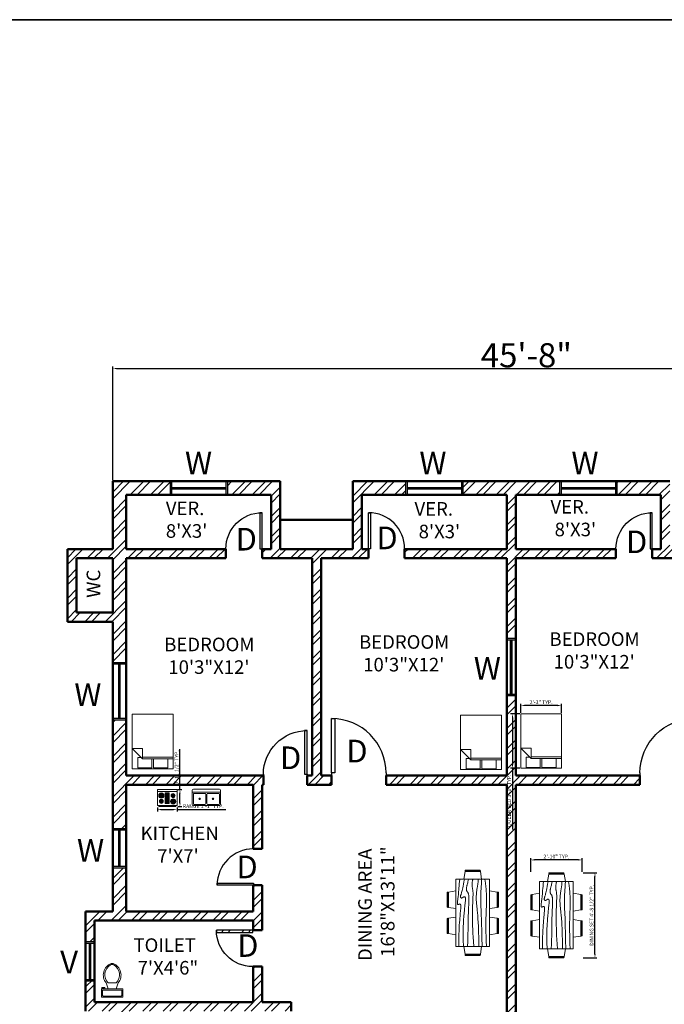
# Model space of a CAD drawing. Units: inches. Extents: x -31485 to -28799, y 18003 to 19130.
# Tile 9 of 15: x -30506 to -30079, y 18478 to 19130. Entities that reach past the tile are written whole.
import ezdxf

# ---------------------------------------------------------------- set-up
doc = ezdxf.new("R2010")
doc.units = ezdxf.units.IN
for name, color, linetype, lineweight in [('A-ANNO-DIMS', 2, 'Continuous', 18), ('A-ANNO-TEXT', 7, 'Continuous', 18), ('A-ANNO-TTLB', 7, 'Continuous', 35), ('A-AREA-IDEN', 7, 'Continuous', 18), ('A-DOOR', 3, 'Continuous', 25), ('A-FLOR-FIXT', 9, 'Continuous', 18), ('A-FURN', 8, 'Continuous', 18), ('A-GLAZ', 4, 'Continuous', 25), ('A-WALL', 7, 'Continuous', 50), ('A-WALL-PATT', 8, 'Continuous', 13)]:
    doc.layers.add(name, color=color, linetype=linetype, lineweight=lineweight)
doc.styles.get("Standard").update_dxf_attribs({"font": 'arial.ttf'})
doc.dimstyles.new('ISO-25', dxfattribs={"dimtxt": 2.5, "dimasz": 2.5, "dimexe": 1.25, "dimexo": 0.625, "dimtad": 1, "dimdec": 0, "dimlunit": 3, "dimtxsty": 'Standard', "dimcen": 2.5, "dimadec": 0, "dimazin": 0, "dimtfac": 1, "dimtdec": 0, "dimtmove": 0, "dimatfit": 3, "dimfxl": 1, "dimarcsym": 0})

# ---------------------------------------------------------------- blocks, each defined once
blk = doc.blocks.new('*U8')
for p, q in [((0, 0), (0, -100)), ((750, 0), (750, -100))]:
    blk.add_line(p, q)
blk.add_lwpolyline([(0, 0), (0, 750), (43.75, 750), (43.75, 0)], close=True)
blk.add_arc((0, 0), 750, 0, 90)
blk = doc.blocks.new('Bed - Queen')
for p, q in [((0, -80.00003), (0, 0)), ((0, 0), (59.99999, 0)), ((59.99999, 0), (59.99999, -80.00003)), ((0, -14.4), (44.8, -14.4)), ((7.99999, -1.2), (28.79998, -1.2)), ((7.99999, -14.4), (7.99999, -1.2)), ((28.79998, -1.2), (28.79998, -14.4)), ((31.19999, -1.2), (51.99999, -1.2)), ((31.19999, -14.4), (31.19999, -1.2)), ((59.99999, -29.6), (44.8, -14.4)), ((44.8, -14.4), (44.8, -29.6)), ((51.99999, -1.2), (51.99999, -16.4)), ((44.8, -16.8), (0, -16.8)), ((51.99999, -16.4), (46.79936, -16.4)), ((44.8, -29.6), (59.99999, -29.6)), ((59.99999, -80.00003), (0, -80.00003))]:
    blk.add_line(p, q)
blk = doc.blocks.new('Range-Oven - 30 in top')
for p, q in [((0, -3), (30, -3)), ((12, -6), (18, -6)), ((13, -20), (13, -6)), ((14, -6), (14, -20)), ((15, -20), (15, -6)), ((16, -6), (16, -20)), ((17, -20), (17, -6)), ((6, -24), (6, -25)), ((8, -25), (8, -24)), ((18, -20), (12, -20)), ((22, -25), (22, -24)), ((24, -24), (24, -25))]:
    blk.add_line(p, q)
for points in [[(0, -24), (0, 0), (30, 0), (30, -24)], [(12, -21), (12, -5), (18, -5), (18, -21)], [(2, -26), (2, -25), (28, -25), (28, -26)]]:
    blk.add_lwpolyline(points, close=True)
for centre, radius in [((6, -9), 4), ((6, -9), 3), ((6, -18), 3), ((6, -9), 2), ((6, -9), 1), ((24, -18), 4), ((24, -9), 3), ((24, -18), 3), ((24, -9), 2), ((24, -9), 1), ((6, -18), 2), ((6, -18), 1), ((24, -18), 2), ((24, -18), 1)]:
    blk.add_circle(centre, radius)
blk = doc.blocks.new('Sink-double - 36 in top')
for p, q in [((-18, -4), (18, -4)), ((-0.75, -18.5), (-0.75, -6.5)), ((0.75, -6.5), (0.75, -18.5))]:
    blk.add_line(p, q)
for points in [[(-16.5, 0), (16.5, 0)], [(-18, -19.5), (-18, -1.5)], [(-16.5, -18.5), (-16.5, -6.5)], [(-15.5, -5.5), (-1.75, -5.5)], [(1.75, -5.5), (15.5, -5.5)], [(16.5, -6.5), (16.5, -18.5)], [(18, -1.5), (18, -19.5)], [(16.5, -21), (-16.5, -21)], [(-1.75, -19.5), (-15.5, -19.5)], [(15.5, -19.5), (1.75, -19.5)]]:
    blk.add_lwpolyline(points)
for centre, radius in [((-8.5, -12.5), 1), ((-8.5, -12.5), 0.5), ((8.5, -12.5), 1), ((8.5, -12.5), 0.5)]:
    blk.add_circle(centre, radius)
for centre, radius, start, end in [((-16.5, -1.5), 1.5, 90, 180), ((16.5, -1.5), 1.5, 0, 90), ((-15.5, -6.5), 1, 90, 180), ((-1.75, -6.5), 1, 0, 90), ((1.75, -6.5), 1, 90, 180), ((15.5, -6.5), 1, 0, 90), ((-16.5, -19.5), 1.5, 180, 270), ((-15.5, -18.5), 1, 180, 270), ((-1.75, -18.5), 1, 270, 0), ((1.75, -18.5), 1, 180, 270), ((15.5, -18.5), 1, 270, 0), ((16.5, -19.5), 1.5, 270, 0)]:
    blk.add_arc(centre, radius, start, end)
blk = doc.blocks.new('Toilet - top')
for p, q in [((-10, -8.5), (-8, -8.5)), ((-10, -9.5), (-10, -8.5)), ((-7, -9.5), (-10, -9.5)), ((-8, -8.5), (-8, -8)), ((-7, -8), (-7, -9.5)), ((-4, -8), (-6, -14)), ((4, -8), (6, -14)), ((9.5, -6), (9.5, -2)), ((4, -14), (-4, -14))]:
    blk.add_line(p, q)
blk.add_lwpolyline([(10.5, -8), (10.5, 0), (-10.5, 0), (-10.5, -8)], close=True)
for points in [[(-9.5, -2), (-9.5, -6)], [(8.5, -1), (-8.5, -1)], [(-8.5, -7), (8.5, -7)]]:
    blk.add_lwpolyline(points)
for centre, radius, start, end in [((-8.62, -1.88), 0.884, 81.8699, 188.1301), ((-8.62, -6.12), 0.884, 171.8699, 278.1301), ((8.62, -1.88), 0.884, 351.8699, 98.1301), ((8.62, -6.12), 0.884, 261.8699, 8.1301), ((3.52, -21.58), 12.17, 141.46911, 247.97143), ((4.2, -21.82), 11.33, 136.36773, 238.94682), ((-3.52, -21.58), 12.17, 292.02843, 38.53071), ((-4.2, -21.82), 11.33, 301.05301, 43.63209), ((0, -27.88), 4, 245.73182, 294.26817), ((0, -29), 4, 254.86053, 285.13947)]:
    blk.add_arc(centre, radius, start, end)
blk = doc.blocks.new('Dining Set - 36 x 72 in.')
for p, q in [((-22.2343, 26.00059), (-23.4847, 17.99762)), ((-22.2304, 26), (-5.7608, 26)), ((-22, 27.5), (-22.1562, 26.50042)), ((-5.8416, 26.5), (-22.1534, 26.5)), ((-22, 27.5), (-6, 27.5)), ((-5.8437, 26.49966), (-6, 27.5)), ((-4.5152, 17.99762), (-5.7655, 25.99926)), ((5.7657, 26.00059), (4.5153, 17.99762)), ((5.7696, 26), (22.2392, 26)), ((6, 27.5), (5.8438, 26.50042)), ((22.1584, 26.5), (5.8466, 26.5)), ((6, 27.5), (22, 27.5)), ((22.1563, 26.49966), (22, 27.5)), ((23.4848, 17.99762), (22.2345, 25.99926)), ((36, 18), (-36, 18)), ((-36, 18), (-36, -18)), ((36, -18), (36, 18)), ((-45.5, 8), (-44.5004, 8.15617)), ((-45.5, 8), (-45.5, -8)), ((-44.5, -8.15843), (-44.5, 8.15338)), ((-44.0006, 8.23428), (-35.9976, 9.48474)), ((-44, 8.23041), (-44, -8.23915)), ((44.0006, 8.23428), (35.9976, 9.48474)), ((44, 8.23041), (44, -8.23915)), ((44.5, -8.15843), (44.5, 8.15338)), ((45.5, 8), (44.5005, 8.15617)), ((45.5, 8), (45.5, -8)), ((-44.4997, -8.15631), (-45.5, -8)), ((-35.9976, -9.48476), (-43.9993, -8.2345)), ((35.9976, -9.48476), (43.9993, -8.2345)), ((44.4997, -8.15631), (45.5, -8)), ((-36, -18), (36, -18)), ((-22.2343, -26.0006), (-23.4847, -17.99762)), ((-4.5152, -17.99762), (-5.7655, -25.99928)), ((5.7657, -26.0006), (4.5153, -17.99762)), ((23.4848, -17.99762), (22.2345, -25.99928)), ((-22.2304, -26), (-5.7608, -26)), ((-22, -27.5), (-22.1562, -26.50044)), ((-5.8416, -26.5), (-22.1534, -26.5)), ((-22, -27.5), (-6, -27.5)), ((-5.8437, -26.49967), (-6, -27.5)), ((5.7696, -26), (22.2392, -26)), ((6, -27.5), (5.8438, -26.50044)), ((22.1584, -26.5), (5.8466, -26.5)), ((6, -27.5), (22, -27.5)), ((22.1563, -26.49967), (22, -27.5))]:
    blk.add_line(p, q)
for points in [[(-36, 15), (-31.1772, 14.97754), (-26.8079, 14.91406), (-22.8538, 14.81543), (-19.276, 14.6875), (-16.0362, 14.53613), (-13.0957, 14.36718), (-10.4159, 14.18652), (-7.9583, 14), (-5.6904, 13.81315), (-3.6035, 13.63021), (-1.6954, 13.45508), (0.0365, 13.29166), (1.5945, 13.14388), (2.9811, 13.01562), (4.1988, 12.9108), (5.25, 12.83333), (6.1393, 12.78613), (6.8802, 12.76823), (7.4883, 12.77767), (7.9792, 12.8125), (8.3685, 12.87077), (8.6719, 12.95052), (8.9049, 13.0498), (9.0833, 13.16666), (9.2205, 13.29899), (9.3216, 13.44401), (9.3895, 13.59879), (9.4271, 13.76041), (9.4373, 13.92594), (9.4232, 14.09245), (9.3875, 14.257), (9.3333, 14.41666), (9.2638, 14.56917), (9.1836, 14.71484), (9.0975, 14.85465), (9.0104, 14.98958), (8.9272, 15.1206), (8.8529, 15.2487), (8.7922, 15.37483), (8.75, 15.5), (8.7305, 15.62467), (8.7344, 15.74739), (8.7617, 15.86621), (8.8125, 15.97916), (8.8867, 16.08431), (8.9844, 16.17968), (9.1055, 16.26334), (9.25, 16.33333), (9.4189, 16.38802), (9.6172, 16.42708), (9.8506, 16.45052), (10.125, 16.45833), (10.4463, 16.45052), (10.8203, 16.42708), (11.2529, 16.38802), (11.75, 16.33333), (12.3184, 16.26318), (12.9694, 16.17838), (13.7151, 16.07991), (14.5677, 15.96875), (15.5395, 15.84586), (16.6426, 15.71224), (17.8893, 15.56884), (19.2917, 15.41666), (20.859, 15.25667), (22.5879, 15.08984), (24.4721, 14.91715), (26.5052, 14.73958), (28.6809, 14.5581), (30.9929, 14.3737), (33.4347, 14.18733), (36, 14)], [(-36, 10), (-28.9766, 10.14274), (-23.1725, 10.20442), (-18.4241, 10.19775), (-14.5677, 10.13541), (-11.4399, 10.03011), (-8.877, 9.89453), (-6.7154, 9.74137), (-4.7917, 9.58333), (-2.9698, 9.43082), (-1.2246, 9.28515), (0.4415, 9.14534), (2.026, 9.01041), (3.5266, 8.87939), (4.9408, 8.7513), (6.266, 8.62516), (7.5, 8.5), (8.6411, 8.37549), (9.6914, 8.2539), (10.6538, 8.13818), (11.5312, 8.03125), (12.3267, 7.93603), (13.043, 7.85547), (13.6831, 7.79248), (14.25, 7.75), (14.7471, 7.7303), (15.1797, 7.73307), (15.5537, 7.75732), (15.875, 7.80208), (16.1494, 7.86637), (16.3828, 7.94922), (16.5811, 8.04964), (16.75, 8.16666), (16.8944, 8.29915), (17.0143, 8.44531), (17.1089, 8.60319), (17.1771, 8.77083), (17.218, 8.94629), (17.2305, 9.1276), (17.2137, 9.31282), (17.1667, 9.5), (17.0895, 9.6875), (16.987, 9.875), (16.8649, 10.0625), (16.7292, 10.25), (16.5856, 10.4375), (16.4401, 10.625), (16.2985, 10.8125), (16.1667, 11), (16.05, 11.18733), (15.9518, 11.3737), (15.8752, 11.5581), (15.8229, 11.73958), (15.798, 11.91715), (15.8034, 12.08984), (15.842, 12.25667), (15.9167, 12.41666), (16.0295, 12.56836), (16.1784, 12.70833), (16.3605, 12.83268), (16.5729, 12.9375), (16.8127, 13.01888), (17.0768, 13.07291), (17.3625, 13.0957), (17.6667, 13.08333), (17.9894, 13.03312), (18.3418, 12.94726), (18.7382, 12.82918), (19.1927, 12.68229), (19.7195, 12.51001), (20.3327, 12.31575), (21.0465, 12.10294), (21.875, 11.875), (22.8357, 11.63354), (23.959, 11.37304), (25.2786, 11.08618), (26.8282, 10.76562), (28.6414, 10.40405), (30.752, 9.99414), (33.1936, 9.52856), (36, 9)], [(-36, 5.5), (-30.7157, 5.3348), (-26.069, 5.20963), (-21.9946, 5.11767), (-18.4271, 5.05208), (-15.3009, 5.00602), (-12.5508, 4.97265), (-10.1112, 4.94515), (-7.9167, 4.91666), (-5.909, 4.88167), (-4.0586, 4.83984), (-2.3429, 4.79215), (-0.7396, 4.73958), (0.7739, 4.6831), (2.22, 4.6237), (3.6213, 4.56233), (5, 4.5), (6.373, 4.43782), (7.7344, 4.3776), (9.0723, 4.32129), (10.375, 4.27083), (11.6309, 4.22819), (12.8281, 4.19531), (13.9551, 4.17415), (15, 4.16666), (15.954, 4.17448), (16.819, 4.19791), (17.6001, 4.23698), (18.3021, 4.29166), (18.9299, 4.36198), (19.4883, 4.44791), (19.9823, 4.54948), (20.4167, 4.66666), (20.7969, 4.79899), (21.1302, 4.94401), (21.4245, 5.09879), (21.6875, 5.26041), (21.9271, 5.42594), (22.1511, 5.59245), (22.3672, 5.757), (22.5834, 5.91666), (22.8065, 6.06868), (23.0404, 6.21093), (23.2879, 6.34147), (23.5521, 6.45833), (23.8358, 6.55957), (24.142, 6.64323), (24.4735, 6.70735), (24.8334, 6.75), (25.2235, 6.76969), (25.642, 6.76692), (26.0858, 6.74267), (26.5521, 6.69791), (27.0379, 6.63362), (27.5404, 6.55078), (28.0565, 6.45036), (28.5834, 6.33333), (29.1242, 6.19987), (29.7071, 6.04687), (30.3661, 5.87044), (31.1354, 5.66666), (32.0493, 5.43164), (33.142, 5.16146), (34.4475, 4.85221), (36, 4.5)], [(-36, -1), (-30.7915, -0.6591), (-26.0195, -0.38216), (-21.6519, -0.16284), (-17.6563, 0.00521), (-14.0005, 0.12833), (-10.6523, 0.21289), (-7.5796, 0.26522), (-4.75, 0.29166), (-2.134, 0.29793), (0.2878, 0.28711), (2.5317, 0.26163), (4.6146, 0.22396), (6.5529, 0.17651), (8.3633, 0.12174), (10.0623, 0.06209), (11.6667, 0), (13.1899, -0.06201), (14.6341, -0.1211), (15.9982, -0.17432), (17.2813, -0.21875), (18.4823, -0.25147), (19.6003, -0.26953), (20.6343, -0.27002), (21.5834, -0.25), (22.4481, -0.20768), (23.2357, -0.14584), (23.9549, -0.06836), (24.6146, 0.02083), (25.2235, 0.11784), (25.7904, 0.21875), (26.3241, 0.31966), (26.8334, 0.41666), (27.3265, 0.50618), (27.8099, 0.58593), (28.2894, 0.65397), (28.7709, 0.70833), (29.2601, 0.74707), (29.763, 0.76823), (30.2855, 0.76985), (30.8334, 0.75), (31.4088, 0.70784), (31.9994, 0.64713), (32.589, 0.57275), (33.1615, 0.48958), (33.7008, 0.4025), (34.1908, 0.3164), (34.6153, 0.23616), (34.9584, 0.16666), (35.2099, 0.11165), (35.3848, 0.07031), (35.504, 0.04069), (35.5886, 0.02083), (35.6594, 0.00879), (35.7377, 0.0026), (35.8442, 0.00032), (36, 0)], [(-36, -6.5), (-27.1843, -6.31267), (-20.084, -6.1263), (-14.469, -5.9419), (-10.1094, -5.76042), (-6.7752, -5.58285), (-4.2363, -5.41016), (-2.2629, -5.24333), (-0.625, -5.08334), (0.8708, -4.93099), (2.2715, -4.78646), (3.5872, -4.64974), (4.8281, -4.52084), (6.0046, -4.39974), (7.127, -4.28646), (8.2053, -4.18099), (9.25, -4.08334), (10.2705, -3.99382), (11.2734, -3.91407), (12.2647, -3.84603), (13.25, -3.79167), (14.2354, -3.75293), (15.2266, -3.73177), (16.2295, -3.73015), (17.25, -3.75), (18.2912, -3.79248), (19.3451, -3.85547), (20.4009, -3.93604), (21.4479, -4.03125), (22.4754, -4.13819), (23.4727, -4.25391), (24.4289, -4.37549), (25.3334, -4.5), (26.1785, -4.62492), (26.9694, -4.74935), (27.7145, -4.87281), (28.4219, -4.99479), (29.1, -5.11483), (29.7572, -5.23242), (30.4016, -5.34709), (31.0417, -5.45834), (31.6837, -5.56437), (32.3262, -5.65821), (32.9658, -5.73153), (33.599, -5.77604), (34.2224, -5.78345), (34.8327, -5.74545), (35.4264, -5.65373), (36, -5.5)], [(-36, -10), (-26.4022, -9.81299), (-18.4675, -9.62891), (-11.9839, -9.45069), (-6.7396, -9.28125), (-2.5226, -9.12354), (0.8789, -8.98047), (3.6769, -8.85498), (6.0833, -8.75), (8.2767, -8.66765), (10.3021, -8.60677), (12.1712, -8.56543), (13.8958, -8.54167), (15.4876, -8.53353), (16.9583, -8.53907), (18.3197, -8.55632), (19.5834, -8.58334), (20.7616, -8.61841), (21.8685, -8.66081), (22.9188, -8.71004), (23.9271, -8.76563), (24.9081, -8.82707), (25.8763, -8.89388), (26.8465, -8.96558), (27.8334, -9.04167), (28.8474, -9.12118), (29.8828, -9.20117), (30.93, -9.27824), (31.9792, -9.34896), (33.0205, -9.40991), (34.0443, -9.45768), (35.0407, -9.48885), (36, -9.5)], [(-36, -14.5), (-30.0881, -14.33513), (-25.0332, -14.21224), (-20.7312, -14.12647), (-17.0781, -14.07292), (-13.97, -14.04671), (-11.3027, -14.04297), (-8.9724, -14.05681), (-6.875, -14.08334), (-4.9224, -14.11833), (-3.0905, -14.16016), (-1.3709, -14.20785), (0.2448, -14.26042), (1.7647, -14.3169), (3.1973, -14.3763), (4.5507, -14.43767), (5.8333, -14.5), (7.0554, -14.5621), (8.235, -14.62175), (9.3922, -14.67652), (10.5469, -14.72396), (11.7192, -14.76164), (12.929, -14.78711), (14.1965, -14.79794), (15.5417, -14.79167), (16.9933, -14.76424), (18.6152, -14.70508), (20.4804, -14.60197), (22.6615, -14.44271), (25.2312, -14.21509), (28.2624, -13.9069), (31.8277, -13.50594), (36, -13)]]:
    blk.add_lwpolyline(points)
blk = doc.blocks.new('*D188')
at = {"layer": 'A-ANNO-DIMS', "color": 0, "lineweight": -2, "transparency": 16777216}
for p, q in [((-30444.21, 18824.74), (-30444.21, 18900.08)), ((-30441.71, 18898.83), (-29898.71, 18898.83)), ((-29896.21, 18824.74), (-29896.21, 18900.08))]:
    blk.add_line(p, q, dxfattribs=at)
at = {"layer": 'A-ANNO-DIMS', "color": 0, "transparency": 16777216}
for points in [[(-30441.71, 18899.25), (-30441.71, 18898.41), (-30444.21, 18898.83)], [(-29898.71, 18899.25), (-29898.71, 18898.41), (-29896.21, 18898.83)]]:
    blk.add_solid(points, dxfattribs=at)
at = {"layer": 'Defpoints', "color": 0, "transparency": 16777216}
for p in [(-29896.21, 18898.83), (-30444.21, 18824.12), (-29896.21, 18824.12)]:
    blk.add_point(p, dxfattribs=at)
at = {"layer": 'A-ANNO-DIMS', "color": 0, "transparency": 16777216, "insert": (-30170.21, 18907.62), "char_height": 2.5, "attachment_point": 5}
blk.add_mtext('{\\H6.4x;45\'-8"}', dxfattribs=at)
blk = doc.blocks.new('WIN-900-W9')
for p, q in [((-29982.21, 18824.12), (-29982.21, 18815.12)), ((-29981.21, 18824.12), (-29981.21, 18815.12)), ((-29981.21, 18820.12), (-29945.21, 18820.12)), ((-29981.21, 18819.62), (-29945.21, 18819.62)), ((-29945.21, 18824.12), (-29945.21, 18815.12)), ((-29944.21, 18824.12), (-29944.21, 18815.12)), ((-29981.21, 18819.12), (-29945.21, 18819.12))]:
    blk.add_line(p, q)
blk = doc.blocks.new('WIN-900-W6')
for p, q in [((-30183.21, 18720.12), (-30177.21, 18720.12)), ((-30183.21, 18719.12), (-30177.21, 18719.12)), ((-30180.71, 18683.12), (-30180.71, 18719.12)), ((-30180.21, 18683.12), (-30180.21, 18719.12)), ((-30179.71, 18683.12), (-30179.71, 18719.12)), ((-30183.21, 18683.12), (-30177.21, 18683.12)), ((-30183.21, 18682.12), (-30177.21, 18682.12))]:
    blk.add_line(p, q)
blk = doc.blocks.new('VENT-600-W9')
for p, q in [((-29896.21, 18594.12), (-29905.21, 18594.12)), ((-29896.21, 18593.12), (-29905.21, 18593.12)), ((-29901.21, 18593.12), (-29901.21, 18569.12)), ((-29900.71, 18593.12), (-29900.71, 18569.12)), ((-29900.21, 18593.12), (-29900.21, 18569.12)), ((-29896.21, 18569.12), (-29905.21, 18569.12)), ((-29896.21, 18568.12), (-29905.21, 18568.12))]:
    blk.add_line(p, q)
blk = doc.blocks.new('VENT-600-W6')
for p, q in [((-29884.21, 18519.12), (-29878.21, 18519.12)), ((-29884.21, 18518.12), (-29878.21, 18518.12)), ((-29881.71, 18494.12), (-29881.71, 18518.12)), ((-29881.21, 18494.12), (-29881.21, 18518.12)), ((-29880.71, 18494.12), (-29880.71, 18518.12)), ((-29884.21, 18494.12), (-29878.21, 18494.12)), ((-29884.21, 18493.12), (-29878.21, 18493.12))]:
    blk.add_line(p, q)
blk = doc.blocks.new('*D218')
at = {"layer": 'A-ANNO-DIMS', "color": 0, "lineweight": -2, "transparency": 16777216}
for p, q in [((-30174.6, 18670.11), (-30180.64, 18670.11)), ((-30179.39, 18667.61), (-30179.39, 18636.49)), ((-30174.6, 18633.99), (-30180.64, 18633.99)), ((-30179.39, 18633.99), (-30179.39, 18593.47))]:
    blk.add_line(p, q, dxfattribs=at)
at = {"layer": 'A-ANNO-DIMS', "color": 0, "transparency": 16777216}
for points in [[(-30179.81, 18667.61), (-30178.98, 18667.61), (-30179.39, 18670.11)], [(-30179.81, 18636.49), (-30178.98, 18636.49), (-30179.39, 18633.99)]]:
    blk.add_solid(points, dxfattribs=at)
at = {"layer": 'Defpoints', "color": 0, "transparency": 16777216}
for p in [(-30173.97, 18670.11), (-30179.39, 18633.99), (-30173.97, 18633.99)]:
    blk.add_point(p, dxfattribs=at)
at = {"layer": 'A-ANNO-DIMS', "color": 0, "transparency": 16777216, "insert": (-30181.39, 18612.48), "char_height": 2.5, "attachment_point": 5, "rotation": 90}
blk.add_mtext('QUEEN BED 3\'-0" TYP.', dxfattribs=at)
blk = doc.blocks.new('*D219')
at = {"layer": 'A-ANNO-DIMS', "color": 0, "lineweight": -2, "transparency": 16777216}
for p, q in [((-30173.97, 18670.73), (-30173.97, 18676.78)), ((-30146.89, 18670.73), (-30146.89, 18676.78)), ((-30149.39, 18675.53), (-30171.47, 18675.53))]:
    blk.add_line(p, q, dxfattribs=at)
at = {"layer": 'A-ANNO-DIMS', "color": 0, "transparency": 16777216}
for points in [[(-30171.47, 18675.94), (-30171.47, 18675.11), (-30173.97, 18675.53)], [(-30149.39, 18675.94), (-30149.39, 18675.11), (-30146.89, 18675.53)]]:
    blk.add_solid(points, dxfattribs=at)
at = {"layer": 'Defpoints', "color": 0, "transparency": 16777216}
for p in [(-30173.97, 18675.53), (-30173.97, 18670.11), (-30146.89, 18670.11)]:
    blk.add_point(p, dxfattribs=at)
at = {"layer": 'A-ANNO-DIMS', "color": 0, "transparency": 16777216, "insert": (-30160.43, 18677.43), "char_height": 2.5, "attachment_point": 5}
blk.add_mtext('2\'-3" TYP.', dxfattribs=at)
blk = doc.blocks.new('*D246')
at = {"layer": 'A-ANNO-DIMS', "color": 0, "lineweight": -2, "transparency": 16777216}
for p, q in [((-30414.63, 18607.93), (-30414.63, 18605.36)), ((-30412.13, 18606.61), (-30404.13, 18606.61)), ((-30401.63, 18607.93), (-30401.63, 18605.36)), ((-30401.63, 18606.61), (-30369.38, 18606.61))]:
    blk.add_line(p, q, dxfattribs=at)
at = {"layer": 'A-ANNO-DIMS', "color": 0, "transparency": 16777216}
for points in [[(-30412.13, 18607.03), (-30412.13, 18606.19), (-30414.63, 18606.61)], [(-30404.13, 18607.03), (-30404.13, 18606.19), (-30401.63, 18606.61)]]:
    blk.add_solid(points, dxfattribs=at)
at = {"layer": 'Defpoints', "color": 0, "transparency": 16777216}
for p in [(-30414.63, 18608.56), (-30401.63, 18608.56), (-30401.63, 18606.61)]:
    blk.add_point(p, dxfattribs=at)
at = {"layer": 'A-ANNO-DIMS', "color": 0, "transparency": 16777216, "insert": (-30384.25, 18608.53), "char_height": 2.5, "attachment_point": 5}
blk.add_mtext('RANGE 1\'-1" TYP.', dxfattribs=at)
blk = doc.blocks.new('*D247')
at = {"layer": 'A-ANNO-DIMS', "color": 0, "lineweight": -2, "transparency": 16777216}
for p, q in [((-30399.68, 18619.83), (-30399.68, 18646.58)), ((-30401, 18619.83), (-30398.43, 18619.83)), ((-30399.68, 18611.06), (-30399.68, 18617.33)), ((-30401, 18608.56), (-30398.43, 18608.56))]:
    blk.add_line(p, q, dxfattribs=at)
at = {"layer": 'A-ANNO-DIMS', "color": 0, "transparency": 16777216}
for points in [[(-30400.09, 18617.33), (-30399.26, 18617.33), (-30399.68, 18619.83)], [(-30400.09, 18611.06), (-30399.26, 18611.06), (-30399.68, 18608.56)]]:
    blk.add_solid(points, dxfattribs=at)
at = {"layer": 'Defpoints', "color": 0, "transparency": 16777216}
for p in [(-30401.63, 18619.83), (-30399.68, 18619.83), (-30401.63, 18608.56)]:
    blk.add_point(p, dxfattribs=at)
at = {"layer": 'A-ANNO-DIMS', "color": 0, "transparency": 16777216, "insert": (-30401.59, 18634.45), "char_height": 2.5, "attachment_point": 5, "rotation": 90}
blk.add_mtext('0\'-11 1/2" TYP.', dxfattribs=at)
blk = doc.blocks.new('*D258')
at = {"layer": 'A-ANNO-DIMS', "color": 0, "lineweight": -2, "transparency": 16777216}
for p, q in [((-30132.6, 18564.8), (-30123.51, 18564.8)), ((-30124.76, 18510.87), (-30124.76, 18562.3)), ((-30132.6, 18508.37), (-30123.51, 18508.37))]:
    blk.add_line(p, q, dxfattribs=at)
at = {"layer": 'A-ANNO-DIMS', "color": 0, "transparency": 16777216}
for points in [[(-30125.17, 18562.3), (-30124.34, 18562.3), (-30124.76, 18564.8)], [(-30125.17, 18510.87), (-30124.34, 18510.87), (-30124.76, 18508.37)]]:
    blk.add_solid(points, dxfattribs=at)
at = {"layer": 'Defpoints', "color": 0, "transparency": 16777216}
for p in [(-30133.22, 18564.8), (-30124.76, 18564.8), (-30133.22, 18508.37)]:
    blk.add_point(p, dxfattribs=at)
at = {"layer": 'A-ANNO-DIMS', "color": 0, "transparency": 16777216, "insert": (-30126.68, 18536.59), "char_height": 2.5, "attachment_point": 5, "rotation": 90}
blk.add_mtext('DINING SET 4\'-8 1/2" TYP.', dxfattribs=at)
blk = doc.blocks.new('*D259')
at = {"layer": 'A-ANNO-DIMS', "color": 0, "lineweight": -2, "transparency": 16777216}
for p, q in [((-30167.33, 18565.43), (-30167.33, 18574.52)), ((-30135.72, 18573.27), (-30164.83, 18573.27)), ((-30133.22, 18565.43), (-30133.22, 18574.52))]:
    blk.add_line(p, q, dxfattribs=at)
at = {"layer": 'A-ANNO-DIMS', "color": 0, "transparency": 16777216}
for points in [[(-30164.83, 18573.68), (-30164.83, 18572.85), (-30167.33, 18573.27)], [(-30135.72, 18573.68), (-30135.72, 18572.85), (-30133.22, 18573.27)]]:
    blk.add_solid(points, dxfattribs=at)
at = {"layer": 'Defpoints', "color": 0, "transparency": 16777216}
for p in [(-30167.33, 18573.27), (-30167.33, 18564.8), (-30133.22, 18564.8)]:
    blk.add_point(p, dxfattribs=at)
at = {"layer": 'A-ANNO-DIMS', "color": 0, "transparency": 16777216, "insert": (-30150.27, 18575.17), "char_height": 2.5, "attachment_point": 5}
blk.add_mtext('2\'-10" TYP.', dxfattribs=at)

msp = doc.modelspace()

# ---------------------------------------------------------------- hatches: boundary and pattern name
at = {"layer": 'A-WALL-PATT'}
h = msp.add_hatch(dxfattribs=at)
h.set_pattern_fill('ANSI32', color=256)
h.paths.add_polyline_path([(-30435.21, 18779.12), (-30435.21, 18815.12), (-30406.21, 18815.12), (-30406.21, 18824.12), (-30444.21, 18824.12), (-30444.21, 18779.12), (-30474.21, 18779.12), (-30474.21, 18731.12), (-30444.21, 18731.12), (-30444.21, 18704.18), (-30435.21, 18704.18), (-30435.21, 18773.12), (-30369.28, 18773.12), (-30369.28, 18779.12)])
h.paths.add_polyline_path([(-30444.21, 18773.12), (-30444.21, 18737.12), (-30468.21, 18737.12), (-30468.21, 18773.12)], flags=16)
h.paths.add_polyline_path([(-30333.21, 18824.12), (-30368.21, 18824.12), (-30368.21, 18815.12), (-30339.21, 18815.12), (-30339.21, 18779.12), (-30345.28, 18779.12), (-30345.28, 18773.12), (-30312.21, 18773.12), (-30312.21, 18629.12), (-30315.41, 18629.12), (-30315.41, 18626.12), (-30315.41, 18623.12), (-30299.19, 18623.12), (-30299.19, 18629.12), (-30306.21, 18629.12), (-30306.21, 18773.12), (-30274.83, 18773.12), (-30274.83, 18779.12), (-30279.21, 18779.12), (-30279.21, 18815.12), (-30250.21, 18815.12), (-30250.21, 18824.12), (-30285.21, 18824.12), (-30285.21, 18779.12), (-30333.21, 18779.12)])
h.paths.add_polyline_path([(-30177.21, 18779.12), (-30177.21, 18815.12), (-30148.21, 18815.12), (-30148.21, 18824.12), (-30212.21, 18824.12), (-30212.21, 18815.12), (-30183.21, 18815.12), (-30183.21, 18779.12), (-30250.83, 18779.12), (-30250.83, 18776.12), (-30250.83, 18773.12), (-30183.21, 18773.12), (-30183.21, 18720.12), (-30177.21, 18720.12), (-30177.21, 18773.12), (-30110.84, 18773.12), (-30110.84, 18779.12)])
h.paths.add_polyline_path([(-30015.86, 18779.12), (-30021.21, 18779.12), (-30021.21, 18815.12), (-29982.21, 18815.12), (-29982.21, 18824.12), (-30027.21, 18824.12), (-30027.21, 18779.12), (-30075.21, 18779.12), (-30075.21, 18824.12), (-30110.21, 18824.12), (-30110.21, 18815.12), (-30081.21, 18815.12), (-30081.21, 18779.12), (-30086.84, 18779.12), (-30086.84, 18776.12), (-30086.84, 18773.12), (-30054.21, 18773.12), (-30054.21, 18629.12), (-30058.98, 18629.12), (-30058.98, 18623.12), (-30045.32, 18623.12), (-30045.32, 18629.12), (-30048.21, 18629.12), (-30048.21, 18773.12), (-30015.86, 18773.12)])
h.paths.add_polyline_path([(-29866.21, 18779.12), (-29896.21, 18779.12), (-29896.21, 18824.12), (-29944.21, 18824.12), (-29944.21, 18815.12), (-29905.21, 18815.12), (-29905.21, 18779.12), (-29991.86, 18779.12), (-29991.86, 18776.12), (-29991.86, 18773.12), (-29905.21, 18773.12), (-29905.21, 18720.12), (-29896.21, 18720.12), (-29896.21, 18731.12), (-29866.21, 18731.12)])
h.paths.add_polyline_path([(-29896.21, 18773.12), (-29872.21, 18773.12), (-29872.21, 18737.12), (-29896.21, 18737.12)], flags=16)
h.paths.add_polyline_path([(-29896.21, 18682.12), (-29905.21, 18682.12), (-29905.21, 18629.12), (-30009.32, 18629.12), (-30009.32, 18626.12), (-30009.32, 18623.12), (-29995.21, 18623.12), (-29995.21, 18573.22), (-29989.21, 18573.22), (-29989.21, 18623.12), (-29905.21, 18623.12), (-29905.21, 18594.12), (-29896.21, 18594.12)])
h.paths.add_polyline_path([(-30094.98, 18629.12), (-30177.21, 18629.12), (-30177.21, 18682.12), (-30183.21, 18682.12), (-30183.21, 18629.12), (-30263.19, 18629.12), (-30263.19, 18626.12), (-30263.19, 18623.12), (-30183.21, 18623.12), (-30183.21, 18425.12), (-30234.21, 18425.12), (-30234.21, 18408.38), (-30228.21, 18408.38), (-30228.21, 18419.12), (-30112.21, 18419.12), (-30112.21, 18406.94), (-30106.21, 18406.94), (-30106.21, 18425.12), (-30177.21, 18425.12), (-30177.21, 18623.12), (-30094.98, 18623.12)])
h.paths.add_polyline_path([(-29896.21, 18568.12), (-29905.21, 18568.12), (-29905.21, 18539.12), (-29989.21, 18539.12), (-29989.21, 18549.22), (-29992.21, 18549.22), (-29995.21, 18549.22), (-29995.21, 18519.45), (-29989.21, 18519.45), (-29989.21, 18533.12), (-29884.21, 18533.12), (-29884.21, 18519.12), (-29878.21, 18519.12), (-29878.21, 18539.12), (-29896.21, 18539.12)])
h.paths.add_polyline_path([(-29878.21, 18493.12), (-29884.21, 18493.12), (-29884.21, 18479.12), (-29989.21, 18479.12), (-29989.21, 18495.45), (-29992.21, 18495.45), (-29995.21, 18495.45), (-29995.21, 18479.12), (-30019.21, 18479.12), (-30019.21, 18473.12), (-29905.21, 18473.12), (-29905.21, 18438.12), (-29896.21, 18438.12), (-29896.21, 18473.12), (-29878.21, 18473.12)])
h.paths.add_polyline_path([(-29896.21, 18400.12), (-29905.21, 18400.12), (-29905.21, 18365.12), (-29952.21, 18365.12), (-29952.21, 18359.12), (-29905.21, 18359.12), (-29905.21, 18309.79), (-29896.21, 18309.79), (-29896.21, 18317.12), (-29866.21, 18317.12), (-29866.21, 18365.12), (-29896.21, 18365.12)])
h.paths.add_polyline_path([(-29896.21, 18359.12), (-29872.21, 18359.12), (-29872.21, 18323.12), (-29896.21, 18323.12)], flags=16)
h.paths.add_polyline_path([(-29990.21, 18365.12), (-30043.21, 18365.12), (-30050.35, 18365.12), (-30050.35, 18359.12), (-29990.21, 18359.12)])
h.paths.add_polyline_path([(-29896.21, 18271.79), (-29905.21, 18271.79), (-29905.21, 18243.12), (-30046.21, 18243.12), (-30046.21, 18315.12), (-30055.46, 18315.12), (-30055.46, 18309.12), (-30052.21, 18309.12), (-30052.21, 18219.12), (-30066.21, 18219.12), (-30066.21, 18213.12), (-30052.21, 18213.12), (-30052.21, 18180.12), (-29993.21, 18180.12), (-29993.21, 18189.12), (-30046.21, 18189.12), (-30046.21, 18237.12), (-29905.21, 18237.12), (-29905.21, 18189.12), (-29955.21, 18189.12), (-29955.21, 18180.12), (-29896.21, 18180.12)])
h.paths.add_polyline_path([(-30092.21, 18219.12), (-30106.21, 18219.12), (-30106.21, 18309.12), (-30079.46, 18309.12), (-30079.46, 18315.12), (-30106.21, 18315.12), (-30106.21, 18359.12), (-30086.35, 18359.12), (-30086.35, 18365.12), (-30106.21, 18365.12), (-30106.21, 18370.94), (-30112.21, 18370.94), (-30112.21, 18189.12), (-30151.21, 18189.12), (-30151.21, 18180.12), (-30106.21, 18180.12), (-30106.21, 18213.12), (-30092.21, 18213.12)])
h.paths.add_polyline_path([(-30189.21, 18189.12), (-30228.21, 18189.12), (-30228.21, 18225.12), (-30234.21, 18225.12), (-30234.21, 18219.12), (-30248.21, 18219.12), (-30248.21, 18213.12), (-30234.21, 18213.12), (-30234.21, 18180.12), (-30189.21, 18180.12)])
h.paths.add_polyline_path([(-30288.21, 18213.12), (-30274.21, 18213.12), (-30274.21, 18219.12), (-30288.21, 18219.12), (-30288.21, 18309.12), (-30285.87, 18309.12), (-30285.87, 18315.12), (-30294.21, 18315.12), (-30294.21, 18243.12), (-30435.21, 18243.12), (-30435.21, 18263.9), (-30444.21, 18263.9), (-30444.21, 18180.12), (-30383.71, 18180.12), (-30383.71, 18189.12), (-30435.21, 18189.12), (-30435.21, 18237.12), (-30294.21, 18237.12), (-30294.21, 18189.12), (-30345.71, 18189.12), (-30345.71, 18180.12), (-30288.21, 18180.12)])
h.paths.add_polyline_path([(-30435.21, 18359.12), (-30388.21, 18359.12), (-30388.21, 18365.12), (-30435.21, 18365.12), (-30435.21, 18400.12), (-30444.21, 18400.12), (-30444.21, 18365.12), (-30474.21, 18365.12), (-30474.21, 18317.12), (-30444.21, 18317.12), (-30444.21, 18301.9), (-30435.21, 18301.9)])
h.paths.add_polyline_path([(-30444.21, 18323.12), (-30468.21, 18323.12), (-30468.21, 18359.12), (-30444.21, 18359.12)], flags=16)
h.paths.add_polyline_path([(-30294.54, 18365.12), (-30297.21, 18365.12), (-30350.21, 18365.12), (-30350.21, 18359.12), (-30294.54, 18359.12)])
h.paths.add_polyline_path([(-30228.21, 18372.38), (-30234.21, 18372.38), (-30234.21, 18365.12), (-30258.54, 18365.12), (-30258.54, 18359.12), (-30234.21, 18359.12), (-30234.21, 18315.12), (-30261.87, 18315.12), (-30261.87, 18309.12), (-30234.21, 18309.12), (-30234.21, 18225.12), (-30228.21, 18225.12)])
h.paths.add_polyline_path([(-30375.49, 18525.25), (-30375.54, 18525.25), (-30375.54, 18526.65), (-30351.51, 18526.65), (-30351.51, 18525.25), (-30375.49, 18525.25, 0.400923), (-30351.21, 18502.63), (-30351.21, 18502.64), (-30345.21, 18502.64), (-30345.21, 18479.12), (-30325.98, 18479.12), (-30325.98, 18473.12), (-30435.21, 18473.12), (-30435.21, 18437.12), (-30439.21, 18437.12), (-30439.21, 18401.12), (-30440.21, 18401.12), (-30440.21, 18437.12), (-30444.21, 18437.12), (-30444.21, 18473.12), (-30462.21, 18473.12), (-30462.21, 18494.12), (-30456.21, 18494.12), (-30456.21, 18479.12), (-30351.21, 18479.12), (-30351.21, 18502.63), (-30351.51, 18502.63, -0.39722)])
h.paths.add_polyline_path([(-30345.21, 18556.53), (-30351.21, 18556.53), (-30351.21, 18539.12), (-30435.21, 18539.12), (-30435.21, 18568.12), (-30444.21, 18568.12), (-30444.21, 18539.12), (-30462.21, 18539.12), (-30462.21, 18519.12), (-30456.21, 18519.12), (-30456.21, 18533.12), (-30351.21, 18533.12), (-30351.21, 18526.64), (-30345.21, 18526.64)])
h.paths.add_polyline_path([(-30344.41, 18629.12), (-30435.21, 18629.12), (-30435.21, 18666.18), (-30444.21, 18666.18), (-30444.21, 18594.12), (-30435.21, 18594.12), (-30435.21, 18623.12), (-30351.21, 18623.12), (-30351.21, 18580.56), (-30347.87, 18580.56), (-30345.21, 18580.53), (-30345.21, 18623.12)])

# ---------------------------------------------------------------- linework, layer by layer
at = {"layer": 'A-ANNO-TTLB'}
msp.add_lwpolyline([(-31485.1, 19129.94), (-28798.64, 19129.94), (-28798.64, 18002.86), (-31485.1, 18002.86)], close=True, dxfattribs=at)
at = {"layer": 'A-WALL'}
for p, q in [((-30444.21, 18824.12), (-30333.21, 18824.12)), ((-30444.21, 18779.12), (-30444.21, 18824.12)), ((-30333.21, 18779.12), (-30333.21, 18824.12)), ((-30285.21, 18779.12), (-30285.21, 18824.12)), ((-30285.21, 18824.12), (-30075.21, 18824.12)), ((-30435.21, 18815.12), (-30339.21, 18815.12)), ((-30435.21, 18779.12), (-30435.21, 18815.12)), ((-30339.21, 18779.12), (-30339.21, 18815.12)), ((-30279.21, 18779.12), (-30279.21, 18815.12)), ((-30279.21, 18815.12), (-30183.21, 18815.12)), ((-30183.21, 18779.12), (-30183.21, 18815.12)), ((-30177.21, 18779.12), (-30177.21, 18815.12)), ((-30177.21, 18815.12), (-30081.21, 18815.12)), ((-30081.21, 18779.12), (-30081.21, 18815.12)), ((-30333.21, 18798.62), (-30285.21, 18798.62)), ((-30474.21, 18779.12), (-30444.21, 18779.12)), ((-30474.21, 18731.12), (-30474.21, 18779.12)), ((-30435.21, 18779.12), (-30369.28, 18779.12)), ((-30369.28, 18779.12), (-30369.28, 18773.12)), ((-30345.28, 18779.12), (-30345.28, 18773.12)), ((-30345.28, 18779.12), (-30339.21, 18779.12)), ((-30333.21, 18779.12), (-30285.21, 18779.12)), ((-30279.21, 18779.12), (-30274.83, 18779.12)), ((-30274.83, 18779.12), (-30274.83, 18773.12)), ((-30250.83, 18779.12), (-30250.83, 18773.12)), ((-30250.83, 18779.12), (-30183.21, 18779.12)), ((-30177.21, 18779.12), (-30110.84, 18779.12)), ((-30110.84, 18779.12), (-30110.84, 18773.12)), ((-30086.84, 18779.12), (-30086.84, 18773.12)), ((-30086.84, 18779.12), (-30081.21, 18779.12)), ((-30468.21, 18773.12), (-30444.21, 18773.12)), ((-30468.21, 18737.12), (-30468.21, 18773.12)), ((-30444.21, 18737.12), (-30444.21, 18773.12)), ((-30435.21, 18773.12), (-30369.28, 18773.12)), ((-30435.21, 18629.12), (-30435.21, 18773.12)), ((-30345.28, 18773.12), (-30312.21, 18773.12)), ((-30312.21, 18629.12), (-30312.21, 18773.12)), ((-30306.21, 18629.12), (-30306.21, 18773.12)), ((-30306.21, 18773.12), (-30274.83, 18773.12)), ((-30250.83, 18773.12), (-30183.21, 18773.12)), ((-30183.21, 18629.12), (-30183.21, 18773.12)), ((-30177.21, 18773.12), (-30110.84, 18773.12)), ((-30177.21, 18629.12), (-30177.21, 18773.12)), ((-30086.84, 18773.12), (-30054.21, 18773.12)), ((-30468.21, 18737.12), (-30444.21, 18737.12)), ((-30474.21, 18731.12), (-30444.21, 18731.12)), ((-30444.21, 18539.12), (-30444.21, 18731.12)), ((-30435.21, 18629.12), (-30344.41, 18629.12)), ((-30344.41, 18623.12), (-30344.41, 18629.12)), ((-30315.41, 18623.12), (-30315.41, 18629.12)), ((-30315.41, 18629.12), (-30312.21, 18629.12)), ((-30306.21, 18629.12), (-30299.19, 18629.12)), ((-30299.19, 18629.12), (-30299.19, 18623.12)), ((-30263.19, 18629.12), (-30263.19, 18623.12)), ((-30263.19, 18629.12), (-30183.21, 18629.12)), ((-30177.21, 18629.12), (-30094.98, 18629.12)), ((-30094.98, 18629.12), (-30094.98, 18623.12)), ((-30435.21, 18623.12), (-30351.21, 18623.12)), ((-30435.21, 18539.12), (-30435.21, 18623.12)), ((-30351.21, 18580.53), (-30351.21, 18623.12)), ((-30345.21, 18623.12), (-30344.41, 18623.12)), ((-30345.21, 18580.53), (-30345.21, 18623.12)), ((-30315.41, 18623.12), (-30299.19, 18623.12)), ((-30263.19, 18623.12), (-30183.21, 18623.12)), ((-30183.21, 18425.12), (-30183.21, 18623.12)), ((-30177.21, 18425.12), (-30177.21, 18623.12)), ((-30177.21, 18623.12), (-30094.98, 18623.12)), ((-30351.21, 18580.53), (-30345.21, 18580.53)), ((-30351.21, 18539.12), (-30351.21, 18556.53)), ((-30351.21, 18556.53), (-30345.21, 18556.53)), ((-30345.21, 18526.64), (-30345.21, 18556.53)), ((-30462.21, 18539.12), (-30444.21, 18539.12)), ((-30462.21, 18473.12), (-30462.21, 18539.12)), ((-30435.21, 18539.12), (-30351.21, 18539.12)), ((-30456.21, 18533.12), (-30351.21, 18533.12)), ((-30456.21, 18479.12), (-30456.21, 18533.12)), ((-30351.21, 18526.64), (-30351.21, 18533.12)), ((-30351.21, 18526.64), (-30345.21, 18526.64)), ((-30351.21, 18479.12), (-30351.21, 18502.64)), ((-30351.21, 18502.64), (-30345.21, 18502.64)), ((-30345.21, 18479.12), (-30345.21, 18502.64)), ((-30456.21, 18479.12), (-30351.21, 18479.12)), ((-30345.21, 18479.12), (-30325.98, 18479.12)), ((-30325.98, 18479.12), (-30325.98, 18473.12))]:
    msp.add_line(p, q, dxfattribs=at)

# ---------------------------------------------------------------- block references
at = {"layer": 'A-DOOR'}
for p, xscale, yscale, zscale in [((-30345.28, 18779.32), -0.0320000000000009, 0.0320000000000009, 0.0320000000000009), ((-30274.83, 18779.32), 0.0320000000000051, 0.0320000000000051, 0.0320000000000051), ((-30086.84, 18779.32), -0.0320000056647152, 0.0320000056647152, 0.0320000056647152), ((-30299.19, 18630.92), 0.0479999999999911, 0.0479999999999911, 0.0479999999999911), ((-30058.98, 18630.92), -0.0479999003599065, 0.0479999003599065, 0.0479999003599065), ((-30315.41, 18629.98), -0.0386666666666677, 0.0386666666666677, 0.0386666666666677)]:
    msp.add_blockref('*U8', p, dxfattribs=dict(at, xscale=xscale, yscale=yscale, zscale=zscale))
for p, xscale, yscale, zscale, rotation in [((-30351.07, 18556.56), 0.0320000000000009, 0.0320000000000009, 0.0320000000000009, 90.00000000000003), ((-30351.51, 18526.65), -0.0320304342918934, 0.0320304342918934, 0.0320304342918934, 90)]:
    msp.add_blockref('*U8', p, dxfattribs=dict(at, xscale=xscale, yscale=yscale, zscale=zscale, rotation=rotation))
at = {"layer": 'A-FLOR-FIXT'}
for name, p, xscale, yscale, zscale in [('Range-Oven - 30 in top', (-30414.63, 18619.83), 0.4333333333333334, 0.4333333333333334, 0.4333333333333334), ('Sink-double - 36 in top', (-30382.19, 18620.25), 0.5208333333333334, 0.5208333333333334, 0.5208333333333334)]:
    msp.add_blockref(name, p, dxfattribs=dict(at, xscale=xscale, yscale=yscale, zscale=zscale))
at = {"layer": 'A-FLOR-FIXT', "xscale": -0.6786300354967684, "yscale": 0.6786300354967684, "zscale": 0.6786300354967684, "rotation": 180}
msp.add_blockref('Toilet - top', (-30444.59, 18482.33), dxfattribs=at)
at = {"layer": 'A-FURN'}
for name, p, xscale, yscale, zscale, rotation in [('Bed - Queen', (-30404.2, 18633.7), 0.4514551267732207, 0.4514551267732207, 0.4514551267732207, 180), ('Bed - Queen', (-30146.89, 18633.99), 0.4514551267732207, 0.4514551267732207, 0.4514551267732207, 180), ('Bed - Queen', (-30186.68, 18633.13), 0.4514551267732207, 0.4514551267732207, 0.4514551267732207, 180), ('Dining Set - 36 x 72 in.', (-30205.71, 18538.22), 0.6200912778687698, 0.6200912778687698, 0.6200912778687698, 90), ('Dining Set - 36 x 72 in.', (-30150.27, 18536.59), 0.6200912778687698, 0.6200912778687698, 0.6200912778687698, 90)]:
    msp.add_blockref(name, p, dxfattribs=dict(at, xscale=xscale, yscale=yscale, zscale=zscale, rotation=rotation))
at = {"layer": 'A-GLAZ'}
for name, p in [('WIN-900-W9', (-424, 0)), ('WIN-900-W9', (-268, 0)), ('WIN-900-W9', (-166, 0)), ('WIN-900-W6', (0, 0)), ('VENT-600-W6', (-578, 0))]:
    msp.add_blockref(name, p, dxfattribs=at)
for name, p, rotation in [('WIN-900-W9', (-11620.09, 48648.38), 90.00000000001339), ('VENT-600-W9', (-60340.41, 37162.23), 180)]:
    msp.add_blockref(name, p, dxfattribs=dict(at, rotation=rotation))

# ---------------------------------------------------------------- texts
at = {"layer": 'A-ANNO-TEXT', "char_height": 15, "attachment_point": 1}
for s, insert in [('{W}', (-30396.36, 18843.7)), ('{W}', (-30241.09, 18843.7)), ('{W}', (-30140.37, 18843.7)), ('{D}', (-30269.54, 18794.1)), ('{D}', (-30362.83, 18793.27)), ('{D}', (-30104.22, 18791.51)), ('{W}', (-30205.04, 18707.74)), ('{W}', (-30469.66, 18690.34)), ('{D}', (-30289.47, 18652.89)), ('{D}', (-30333.4, 18648.43)), ('{W}', (-30467.87, 18587.04)), ('{D}', (-30362.26, 18576.11)), ('{D}', (-30361.76, 18524.05)), ('{V}', (-30479, 18513.07))]:
    msp.add_mtext_dynamic_manual_height_columns(s, width=1155.9407, gutter_width=12.5, heights=[0], dxfattribs=dict(at, insert=insert))
at = {"layer": 'A-AREA-IDEN', "char_height": 9, "attachment_point": 1}
for s, insert in [("{VER.\\P8'X3'}", (-30409.03, 18810.7)), ("{    VER.\\P     8'X3'}", (-30255.3, 18810.36)), ("{      VER.\\P       8'X3'}", (-30170.73, 18811.7)), ('{BEDROOM\\P 10\'3"X12\'}', (-30281.04, 18722.16)), ('{BEDROOM\\P 10\'3"X12\'}', (-30154.9, 18724.05)), ('{BEDROOM\\P 10\'3"X12\'}', (-30410.1, 18720.51)), ("{ KITCHEN\\P     7'X7'}", (-30428.49, 18595.39)), ('{   TOILET\\P    7\'X4\'6"}', (-30438.72, 18521.32))]:
    msp.add_mtext_dynamic_manual_height_columns(s, width=1354.6859, gutter_width=12.5, heights=[0], dxfattribs=dict(at, insert=insert))
at = {"layer": 'A-AREA-IDEN', "char_height": 9, "attachment_point": 1, "rotation": 90}
for s, insert in [('{WC}', (-30461.5, 18746.93)), ('{DINING AREA\\P 16\'8"X13\'11"}', (-30281.58, 18506.3))]:
    msp.add_mtext_dynamic_manual_height_columns(s, width=1354.6859, gutter_width=12.5, heights=[0], dxfattribs=dict(at, insert=insert))

# ---------------------------------------------------------------- dimensions: what is measured, and where the dimension line sits
at = {"layer": 'A-ANNO-DIMS'}
for base, p1, p2, text, override, picture, middle in [((-29896.21, 18898.83), (-30444.21, 18824.12), (-29896.21, 18824.12), '{\\H6.4x;<>}', {"dimclrd": 0, "dimclre": 0, "dimclrt": 0}, '*D188', (-30170.21, 18907.62)), ((-30401.63, 18606.61), (-30414.63, 18608.56), (-30401.63, 18608.56), 'RANGE <> TYP.', {"dimdec": 1, "dimlfac": 1, "dimrnd": 0, "dimzin": 1, "dimdsep": 46, "dimlunit": 4, "dimfrac": 2}, '*D246', (-30384.25, 18608.53))]:
    dim = msp.add_linear_dim(base=base, p1=p1, p2=p2, text=text, dimstyle='ISO-25', override=override, dxfattribs=at)
    dim.commit()
    dim.dimension.update_dxf_attribs({"geometry": picture, "text_midpoint": middle})
for base, p1, p2, angle, text, picture, middle in [((-30173.97, 18675.53), (-30146.89, 18670.11), (-30173.97, 18670.11), 180, '<> TYP.', '*D219', (-30160.43, 18677.43)), ((-30179.39, 18633.99), (-30173.97, 18670.11), (-30173.97, 18633.99), 270, 'QUEEN BED <> TYP.', '*D218', (-30181.39, 18612.48)), ((-30399.68, 18619.83), (-30401.63, 18608.56), (-30401.63, 18619.83), 90, '<> TYP.', '*D247', (-30401.59, 18634.45)), ((-30167.33, 18573.27), (-30133.22, 18564.8), (-30167.33, 18564.8), 180, '<> TYP.', '*D259', (-30150.27, 18575.17)), ((-30124.76, 18564.8), (-30133.22, 18508.37), (-30133.22, 18564.8), 90, 'DINING SET <> TYP.', '*D258', (-30126.68, 18536.59))]:
    dim = msp.add_linear_dim(base=base, p1=p1, p2=p2, angle=angle, text=text, dimstyle='ISO-25', override={"dimdec": 1, "dimlfac": 1, "dimrnd": 0, "dimzin": 1, "dimdsep": 46, "dimlunit": 4, "dimfrac": 2}, dxfattribs=at)
    dim.commit()
    dim.dimension.update_dxf_attribs({"geometry": picture, "text_midpoint": middle})

doc.saveas('drawing.dxf')
